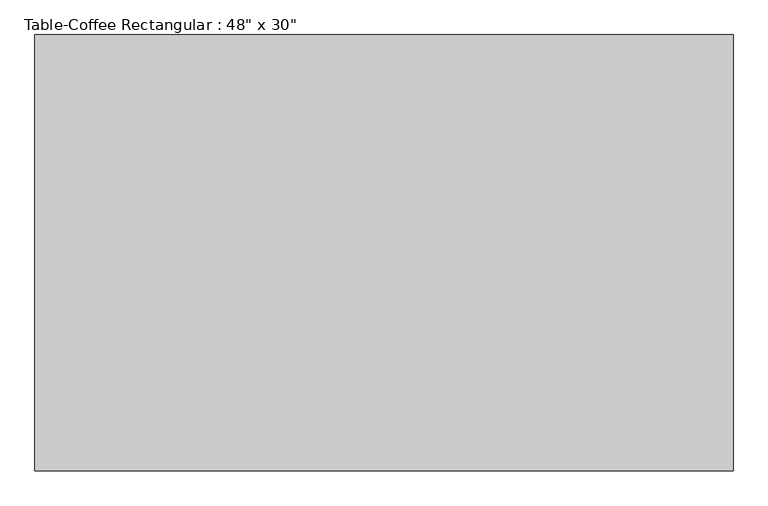
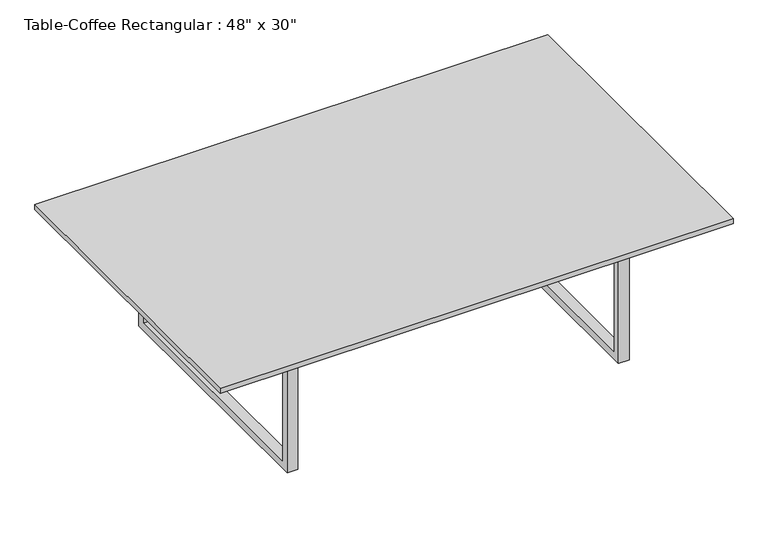
"""IFC4 building model written with IfcOpenShell, lengths in millimetres: furniture geometry."""

from ifc_helpers import new_model, si_unit, frame, origin, place, context, project, spatial, polyline, outline, extrude, source, transform, mapped, element, save


def furniture_acc2807d(model_context):
    return source(origin(), model_context, "Body", "SweptSolid", [
        extrude(outline(polyline([(1222.9336303, 750.6108318), (1222.9336303, -11.3891682), (3.7336303, -11.3891682), (3.7336303, 750.6108318), (1222.9336303, 750.6108318)])), frame((0.0, 0.0, 317.5), z_axis=(0.0, 0.0, 1.0), x_axis=(1.0, 0.0, 0.0)), (0.0, 0.0, 1.0), 12.7),
        extrude(outline(polyline([(64.8108318, 317.5), (674.4108318, 317.5), (674.4108318, 0.0), (64.8108318, 0.0), (64.8108318, 317.5)]), holes=[polyline([(83.8608318, 298.45), (83.8608318, 19.05), (655.3608318, 19.05), (655.3608318, 298.45), (83.8608318, 298.45)])]), frame((206.9336303, 0.0, 0.0), z_axis=(1.0, 0.0, 0.0), x_axis=(0.0, 1.0, 0.0)), (0.0, 0.0, 1.0), 25.4),
        extrude(outline(polyline([(64.8108318, 317.5), (674.4108318, 317.5), (674.4108318, 0.0), (64.8108318, 0.0), (64.8108318, 317.5)]), holes=[polyline([(83.8608318, 298.45), (83.8608318, 19.05), (655.3608318, 19.05), (655.3608318, 298.45), (83.8608318, 298.45)])]), frame((994.3336303, 0.0, 0.0), z_axis=(1.0, 0.0, 0.0), x_axis=(0.0, 1.0, 0.0)), (0.0, 0.0, 1.0), 25.4),
        extrude(outline(polyline([(994.3336303, 379.1358318), (994.3336303, 360.0858318), (232.3336303, 360.0858318), (232.3336303, 379.1358318), (994.3336303, 379.1358318)])), frame((0.0, 0.0, 298.45), z_axis=(0.0, 0.0, 1.0), x_axis=(1.0, 0.0, 0.0)), (0.0, 0.0, 1.0), 19.05),
    ])


if __name__ == "__main__":
    model = new_model("IFC4")
    model_context = context("Model", 3, world=origin())
    ifc_project = project(units=[si_unit("LENGTHUNIT", "METRE", prefix="MILLI")], contexts=[model_context])
    site = spatial("IfcSite", under=ifc_project)
    building = spatial("IfcBuilding", under=site)
    placement = place(None, origin())
    furniture_shape = furniture_acc2807d(model_context)
    element("IfcFurniture", 1, ObjectType="Table-Coffee Rectangular : 48\" x 30\"", at=placement, inside=building, context=model_context, shape_type="MappedRepresentation", body=[
        mapped(furniture_shape, transform((0.0, 0.0, 0.0), x_axis=(1.0, 0.0, 0.0), y_axis=(0.0, 1.0, 0.0), z_axis=(0.0, 0.0, 1.0))),
    ])
    save(model, "model.ifc")

# Revit data of these elements
# Type "Table-Coffee Rectangular : 48\" x 30\""
#   Assembly Code = "E2020200"
#   Height = 1' - 1"
#   Length = 4' - 0"
#   Width = 2' - 6"
#   Base Material = Metal - Chrome
#   Table Top Material = Glass - Clear, Grey
#   Default Elevation = 0
# Element 1 (IfcFurniture, "Table-Coffee Rectangular : 48\" x 30\"")
#   Materials on its faces: "Metal - Chrome", "Glass - Clear, Grey"
# Materials
#   "Metal - Chrome": class "Metal", colour RGB 247 247 247, transparency 0
#   "Glass - Clear, Grey": colour RGB 252 255 255, transparency 0.64
